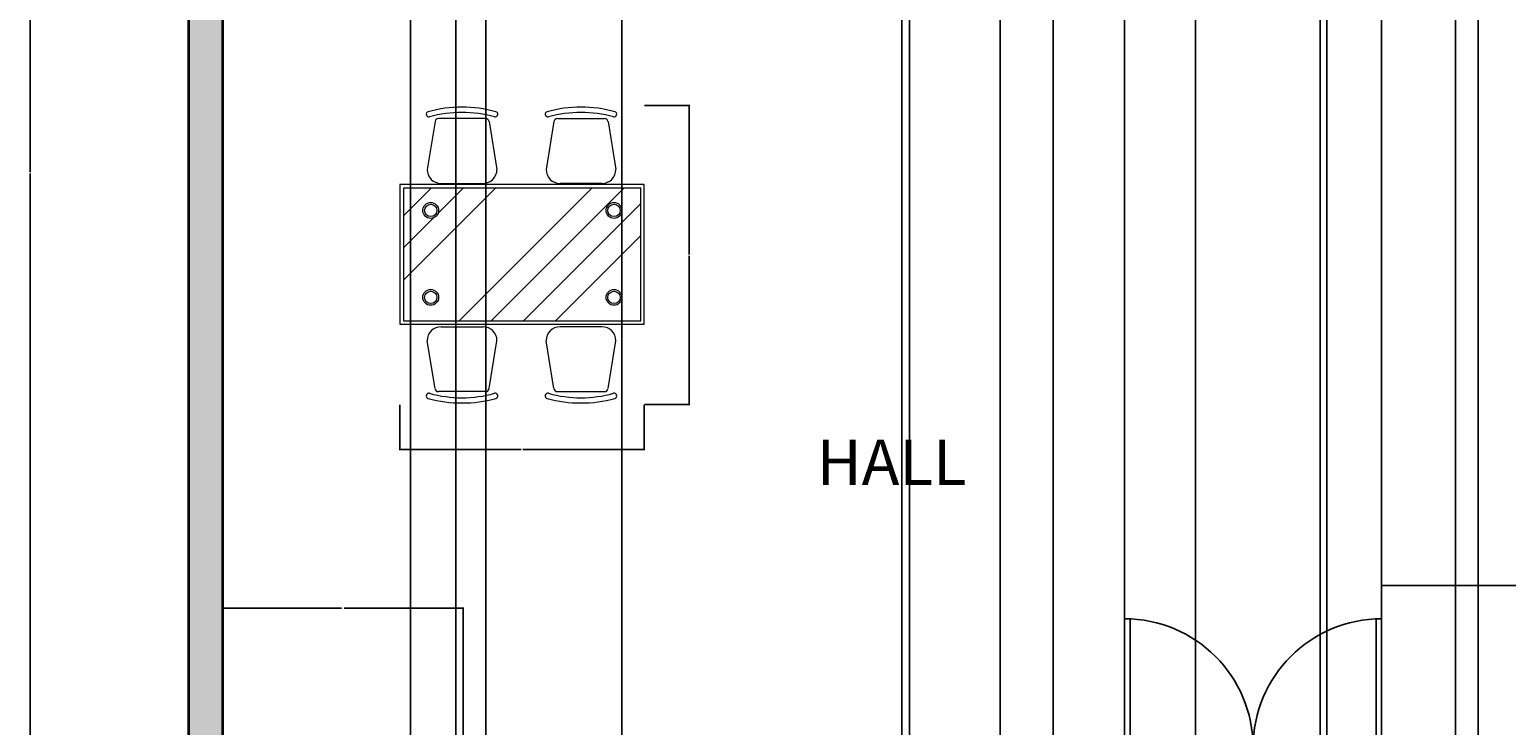
# Model space of a CAD drawing. Units: inches. Extents: x -89 to 661, y -827 to 77.
# Tile 2 of 5: x -44 to 347, y -523 to -339. Entities that reach past the tile are written whole.
import ezdxf

# ---------------------------------------------------------------- set-up
doc = ezdxf.new("R2010")
doc.units = ezdxf.units.IN
doc.header["$MEASUREMENT"] = 0
for name, color, linetype, lineweight in [('A-ANNO-DIMS', 2, 'Continuous', 18), ('A-AREA-IDEN', 7, 'Continuous', 18), ('A-FURN', 34, 'Continuous', 18), ('A-WALL', 7, 'Continuous', 35), ('A-WALL-PATT', 30, 'Continuous', 13), ('DOOR', 5, 'Continuous', 25)]:
    doc.layers.add(name, color=color, linetype=linetype, lineweight=lineweight)
doc.styles.get("Standard").update_dxf_attribs({"font": 'arial.ttf'})
doc.dimstyles.get("Standard").update_dxf_attribs({"dimtxt": 0.18, "dimasz": 0.18, "dimexe": 0.18, "dimexo": 0.0625, "dimgap": 0.09, "dimtad": 0, "dimtih": 1, "dimtoh": 1, "dimdec": 4, "dimzin": 0, "dimdsep": 46, "dimtxsty": 'Standard', "dimcen": 0.09, "dimadec": 0, "dimazin": 0, "dimtfac": 1, "dimtdec": 4, "dimtofl": 0, "dimtmove": 0, "dimatfit": 3, "dimfxl": 1, "dimtolj": 1, "dimtzin": 0, "dimarcsym": 0})

# ---------------------------------------------------------------- blocks, each defined once
blk = doc.blocks.new('*U7')
for p, q in [((0, 0), (0, -6)), ((40, 0), (40, -6))]:
    blk.add_line(p, q)
blk.add_lwpolyline([(0, 0), (0, 40), (1.75, 40), (1.75, 0)], close=True)
blk.add_arc((0, 0), 40, 0, 90)
blk = doc.blocks.new('A$C0FD55737')
for p, q in [((0.2013, 1.6134), (0.1562, 1.3384)), ((0.4912, 1.6302), (0.2211, 1.6302)), ((0.511, 1.6134), (0.5562, 1.3384)), ((0.8828, 1.6134), (0.8376, 1.3384)), ((0.9026, 1.6302), (1.1727, 1.6302)), ((1.1925, 1.6134), (1.2376, 1.3384)), ((0, 1.2513), (0, 0.4513)), ((1.4, 1.2513), (0, 1.2513)), ((0.02, 1.0725), (0.1788, 1.2313)), ((0.02, 0.7043), (0.547, 1.2313)), ((1.38, 1.2313), (0.02, 1.2313)), ((0.02, 1.2313), (0.02, 0.4713)), ((0.2189, 1.0873), (0.3629, 1.2313)), ((0.2362, 1.2584), (0.4762, 1.2584)), ((0.3393, 0.4713), (1.0993, 1.2313)), ((0.5234, 0.4713), (1.2834, 1.2313)), ((1.1576, 1.2584), (0.9176, 1.2584)), ((1.38, 0.4713), (1.38, 1.2313)), ((1.4, 0.4513), (1.4, 1.2513)), ((0.7074, 0.4713), (1.38, 1.1438)), ((0.02, 0.8884), (0.1931, 1.0614)), ((0.8915, 0.4713), (1.38, 0.9597)), ((0, 0.4513), (1.4, 0.4513)), ((0.02, 0.4713), (1.38, 0.4713)), ((0.2362, 0.4371), (0.4762, 0.4371)), ((1.1576, 0.4371), (0.9176, 0.4371)), ((0.2013, 0.0821), (0.1562, 0.3571)), ((0.511, 0.0821), (0.5562, 0.3571)), ((0.8828, 0.0821), (0.8376, 0.3571)), ((1.1925, 0.0821), (1.2376, 0.3571)), ((0.4912, 0.0653), (0.2211, 0.0653)), ((0.9026, 0.0653), (1.1727, 0.0653))]:
    blk.add_line(p, q)
for centre, radius in [((0.1766, 1.1037), 0.0454), ((0.1766, 1.1037), 0.0354), ((1.227, 1.1037), 0.0454), ((1.227, 1.1037), 0.0354), ((0.1766, 0.6052), 0.0454), ((0.1766, 0.6052), 0.0354), ((1.227, 0.6052), 0.0454), ((1.227, 0.6052), 0.0354)]:
    blk.add_circle(centre, radius)
for centre, radius, start, end in [((0.3562, 0.9712), 0.7243, 74.47014, 105.57697), ((1.0376, 0.9712), 0.7243, 74.42303, 105.52986), ((0.1662, 1.6546), 0.015, 105.49005, 284.28424), ((0.3562, 0.9716), 0.6939, 74.43245, 105.56755), ((0.2211, 1.6102), 0.02, 90, 170.67171), ((0.4912, 1.6102), 0.02, 9.32829, 90), ((0.5461, 1.6546), 0.015, 255.71576, 74.50995), ((0.8477, 1.6546), 0.015, 105.49005, 284.28424), ((1.0376, 0.9716), 0.6939, 74.43245, 105.56755), ((0.9026, 1.6102), 0.02, 90, 170.67171), ((1.1727, 1.6102), 0.02, 9.32829, 90), ((1.2276, 1.6546), 0.015, 255.71576, 74.50995), ((0.2362, 1.3384), 0.08, 180, 270), ((0.4762, 1.3384), 0.08, 270, 0), ((0.9176, 1.3384), 0.08, 180, 270), ((1.1576, 1.3384), 0.08, 270, 0), ((0.2362, 0.3571), 0.08, 90, 180), ((0.4762, 0.3571), 0.08, 0, 90), ((0.9176, 0.3571), 0.08, 90, 180), ((1.1576, 0.3571), 0.08, 0, 90), ((0.1662, 0.0409), 0.015, 75.71576, 254.50995), ((0.3562, 0.7243), 0.7243, 254.42303, 285.52986), ((0.3562, 0.7239), 0.6939, 254.43245, 285.56755), ((0.2211, 0.0853), 0.02, 189.32829, 270), ((0.4912, 0.0853), 0.02, 270, 350.67171), ((0.5461, 0.0409), 0.015, 285.49005, 104.28424), ((0.8477, 0.0409), 0.015, 75.71576, 254.50995), ((1.0376, 0.7243), 0.7243, 254.47014, 285.57697), ((1.0376, 0.7239), 0.6939, 254.43245, 285.56755), ((0.9026, 0.0853), 0.02, 189.32829, 270), ((1.1727, 0.0853), 0.02, 270, 350.67171), ((1.2276, 0.0409), 0.015, 285.49005, 104.28424)]:
    blk.add_arc(centre, radius, start, end)
blk = doc.blocks.new('*D25')
at = {"layer": 'A-ANNO-DIMS', "color": 0, "lineweight": -2, "transparency": 16777216}
for p, q in [((118.73, -359.12), (130.71, -359.12)), ((130.53, -359.3), (130.53, -398.47)), ((130.53, -438), (130.53, -398.84)), ((118.73, -438.18), (130.71, -438.18))]:
    blk.add_line(p, q, dxfattribs=at)
at = {"layer": 'A-ANNO-DIMS', "color": 0, "transparency": 16777216}
for points in [[(130.5, -359.3), (130.56, -359.3), (130.53, -359.12)], [(130.5, -438), (130.56, -438), (130.53, -438.18)]]:
    blk.add_solid(points, dxfattribs=at)
at = {"layer": 'Defpoints', "color": 0, "transparency": 16777216}
for p in [(118.67, -359.12), (130.53, -359.12), (118.67, -438.18)]:
    blk.add_point(p, dxfattribs=at)
at = {"layer": 'A-ANNO-DIMS', "color": 0, "transparency": 16777216, "insert": (130.53, -398.65), "char_height": 0.18, "attachment_point": 5}
blk.add_mtext('\\A1;DINING SET 79', dxfattribs=at)
blk = doc.blocks.new('*D26')
at = {"layer": 'A-ANNO-DIMS', "color": 0, "lineweight": -2, "transparency": 16777216}
for p, q in [((54.06, -438.25), (54.06, -450.22)), ((118.67, -438.25), (118.67, -450.22)), ((54.24, -450.04), (86.15, -450.04)), ((118.49, -450.04), (86.59, -450.04))]:
    blk.add_line(p, q, dxfattribs=at)
at = {"layer": 'A-ANNO-DIMS', "color": 0, "transparency": 16777216}
for points in [[(54.24, -450.01), (54.24, -450.07), (54.06, -450.04)], [(118.49, -450.01), (118.49, -450.07), (118.67, -450.04)]]:
    blk.add_solid(points, dxfattribs=at)
at = {"layer": 'Defpoints', "color": 0, "transparency": 16777216}
for p in [(54.06, -438.18), (118.67, -438.18), (118.67, -450.04)]:
    blk.add_point(p, dxfattribs=at)
at = {"layer": 'A-ANNO-DIMS', "color": 0, "transparency": 16777216, "insert": (86.37, -450.04), "char_height": 0.18, "attachment_point": 5}
blk.add_mtext('\\A1;65', dxfattribs=at)
blk = doc.blocks.new('*D32')
at = {"layer": 'A-ANNO-DIMS', "color": 0, "lineweight": -2, "transparency": 16777216}
for p, q in [((-1.88, 29.06), (-43.85, 29.06)), ((-43.67, 28.88), (-43.67, -376.76)), ((-43.67, -782.76), (-43.67, -377.12)), ((-1.88, -782.94), (-43.85, -782.94))]:
    blk.add_line(p, q, dxfattribs=at)
at = {"layer": 'A-ANNO-DIMS', "color": 0, "transparency": 16777216}
for points in [[(-43.7, 28.88), (-43.64, 28.88), (-43.67, 29.06)], [(-43.7, -782.76), (-43.64, -782.76), (-43.67, -782.94)]]:
    blk.add_solid(points, dxfattribs=at)
at = {"layer": 'Defpoints', "color": 0, "transparency": 16777216}
for p in [(-43.67, 29.06), (-1.81, 29.06), (-1.81, -782.94)]:
    blk.add_point(p, dxfattribs=at)
at = {"layer": 'A-ANNO-DIMS', "color": 0, "transparency": 16777216, "insert": (-43.67, -376.94), "char_height": 0.18, "attachment_point": 5}
blk.add_mtext('\\A1;812', dxfattribs=at)
blk = doc.blocks.new('*D44')
at = {"layer": 'A-ANNO-DIMS', "color": 0, "lineweight": -2, "transparency": 16777216}
for p, q in [((299.19, -34), (299.19, -826.85)), ((333.19, -34), (333.19, -826.85)), ((299.37, -826.67), (315.97, -826.67)), ((333.01, -826.67), (316.4, -826.67))]:
    blk.add_line(p, q, dxfattribs=at)
at = {"layer": 'A-ANNO-DIMS', "color": 0, "transparency": 16777216}
for points in [[(299.37, -826.64), (299.37, -826.7), (299.19, -826.67)], [(333.01, -826.64), (333.01, -826.7), (333.19, -826.67)]]:
    blk.add_solid(points, dxfattribs=at)
at = {"layer": 'Defpoints', "color": 0, "transparency": 16777216}
for p in [(299.19, -33.94), (333.19, -33.94), (333.19, -826.67)]:
    blk.add_point(p, dxfattribs=at)
at = {"layer": 'A-ANNO-DIMS', "color": 0, "transparency": 16777216, "insert": (316.19, -826.67), "char_height": 0.18, "attachment_point": 5}
blk.add_mtext('\\A1;34', dxfattribs=at)
blk = doc.blocks.new('*D46')
at = {"layer": 'A-ANNO-DIMS', "color": 0, "lineweight": -2, "transparency": 16777216}
for p, q in [((333.19, -34), (333.19, -826.85)), ((339.19, -34), (339.19, -826.85)), ((333.37, -826.67), (336.04, -826.67)), ((339.01, -826.67), (336.34, -826.67))]:
    blk.add_line(p, q, dxfattribs=at)
at = {"layer": 'A-ANNO-DIMS', "color": 0, "transparency": 16777216}
for points in [[(333.37, -826.64), (333.37, -826.7), (333.19, -826.67)], [(339.01, -826.64), (339.01, -826.7), (339.19, -826.67)]]:
    blk.add_solid(points, dxfattribs=at)
at = {"layer": 'Defpoints', "color": 0, "transparency": 16777216}
for p in [(333.19, -33.94), (339.19, -33.94), (339.19, -826.67)]:
    blk.add_point(p, dxfattribs=at)
at = {"layer": 'A-ANNO-DIMS', "color": 0, "transparency": 16777216, "insert": (336.19, -826.67), "char_height": 0.18, "attachment_point": 5}
blk.add_mtext('\\A1;6', dxfattribs=at)
blk = doc.blocks.new('*D48')
at = {"layer": 'A-ANNO-DIMS', "color": 0, "lineweight": -2, "transparency": 16777216}
for p, q in [((297.44, 2.03), (297.44, -826.85)), ((264.44, -8.47), (264.44, -826.85)), ((264.62, -826.67), (280.72, -826.67)), ((297.26, -826.67), (281.15, -826.67))]:
    blk.add_line(p, q, dxfattribs=at)
at = {"layer": 'A-ANNO-DIMS', "color": 0, "transparency": 16777216}
for points in [[(264.62, -826.64), (264.62, -826.7), (264.44, -826.67)], [(297.26, -826.64), (297.26, -826.7), (297.44, -826.67)]]:
    blk.add_solid(points, dxfattribs=at)
at = {"layer": 'Defpoints', "color": 0, "transparency": 16777216}
for p in [(297.44, 2.09), (264.44, -8.41), (297.44, -826.67)]:
    blk.add_point(p, dxfattribs=at)
at = {"layer": 'A-ANNO-DIMS', "color": 0, "transparency": 16777216, "insert": (280.94, -826.67), "char_height": 0.18, "attachment_point": 5}
blk.add_mtext('\\A1;33', dxfattribs=at)
blk = doc.blocks.new('*D55')
at = {"layer": 'A-ANNO-DIMS', "color": 0, "lineweight": -2, "transparency": 16777216}
for p, q in [((56.84, -267), (56.84, -826.85)), ((68.84, -267), (68.84, -826.85)), ((57.02, -826.67), (62.63, -826.67)), ((68.66, -826.67), (63.05, -826.67))]:
    blk.add_line(p, q, dxfattribs=at)
at = {"layer": 'A-ANNO-DIMS', "color": 0, "transparency": 16777216}
for points in [[(57.02, -826.64), (57.02, -826.7), (56.84, -826.67)], [(68.66, -826.64), (68.66, -826.7), (68.84, -826.67)]]:
    blk.add_solid(points, dxfattribs=at)
at = {"layer": 'Defpoints', "color": 0, "transparency": 16777216}
for p in [(56.84, -266.94), (68.84, -266.94), (68.84, -826.67)]:
    blk.add_point(p, dxfattribs=at)
at = {"layer": 'A-ANNO-DIMS', "color": 0, "transparency": 16777216, "insert": (62.84, -826.67), "char_height": 0.18, "attachment_point": 5}
blk.add_mtext('\\A1;12', dxfattribs=at)
blk = doc.blocks.new('*D56')
at = {"layer": 'A-ANNO-DIMS', "color": 0, "lineweight": -2, "transparency": 16777216}
for p, q in [((188.84, -312), (188.84, -826.85)), ((212.84, -318), (212.84, -826.85)), ((189.02, -826.67), (200.62, -826.67)), ((212.66, -826.67), (201.06, -826.67))]:
    blk.add_line(p, q, dxfattribs=at)
at = {"layer": 'A-ANNO-DIMS', "color": 0, "transparency": 16777216}
for points in [[(189.02, -826.64), (189.02, -826.7), (188.84, -826.67)], [(212.66, -826.64), (212.66, -826.7), (212.84, -826.67)]]:
    blk.add_solid(points, dxfattribs=at)
at = {"layer": 'Defpoints', "color": 0, "transparency": 16777216}
for p in [(188.84, -311.94), (212.84, -317.94), (212.84, -826.67)]:
    blk.add_point(p, dxfattribs=at)
at = {"layer": 'A-ANNO-DIMS', "color": 0, "transparency": 16777216, "insert": (200.84, -826.67), "char_height": 0.18, "attachment_point": 5}
blk.add_mtext('\\A1;24', dxfattribs=at)
blk = doc.blocks.new('*D61')
at = {"layer": 'A-ANNO-DIMS', "color": 0, "lineweight": -2, "transparency": 16777216}
for p, q in [((245.68, -494.78), (245.68, 77.13)), ((245.86, 76.95), (279.46, 76.95)), ((313.5, 76.95), (279.9, 76.95)), ((313.68, -494.78), (313.68, 77.13))]:
    blk.add_line(p, q, dxfattribs=at)
at = {"layer": 'A-ANNO-DIMS', "color": 0, "transparency": 16777216}
for points in [[(245.86, 76.98), (245.86, 76.92), (245.68, 76.95)], [(313.5, 76.98), (313.5, 76.92), (313.68, 76.95)]]:
    blk.add_solid(points, dxfattribs=at)
at = {"layer": 'Defpoints', "color": 0, "transparency": 16777216}
for p in [(313.68, 76.95), (245.68, -494.84), (313.68, -494.84)]:
    blk.add_point(p, dxfattribs=at)
at = {"layer": 'A-ANNO-DIMS', "color": 0, "transparency": 16777216, "insert": (279.68, 76.95), "char_height": 0.18, "attachment_point": 5}
blk.add_mtext('\\A1;68', dxfattribs=at)
blk = doc.blocks.new('*D62')
at = {"layer": 'A-ANNO-DIMS', "color": 0, "lineweight": -2, "transparency": 16777216}
for p, q in [((186.79, -527.88), (186.79, 77.13)), ((186.97, 76.95), (206.57, 76.95)), ((226.61, 76.95), (207.01, 76.95)), ((226.79, -527.88), (226.79, 77.13))]:
    blk.add_line(p, q, dxfattribs=at)
at = {"layer": 'A-ANNO-DIMS', "color": 0, "transparency": 16777216}
for points in [[(186.97, 76.98), (186.97, 76.92), (186.79, 76.95)], [(226.61, 76.98), (226.61, 76.92), (226.79, 76.95)]]:
    blk.add_solid(points, dxfattribs=at)
at = {"layer": 'Defpoints', "color": 0, "transparency": 16777216}
for p in [(226.79, 76.95), (186.79, -527.94), (226.79, -527.94)]:
    blk.add_point(p, dxfattribs=at)
at = {"layer": 'A-ANNO-DIMS', "color": 0, "transparency": 16777216, "insert": (206.79, 76.95), "char_height": 0.18, "attachment_point": 5}
blk.add_mtext('\\A1;40', dxfattribs=at)
blk = doc.blocks.new('*D63')
at = {"layer": 'A-ANNO-DIMS', "color": 0, "lineweight": -2, "transparency": 16777216}
for p, q in [((7.19, -533.88), (7.19, -491.9)), ((7.37, -492.08), (38.66, -492.08)), ((70.61, -492.08), (39.31, -492.08)), ((70.79, -533.88), (70.79, -491.9))]:
    blk.add_line(p, q, dxfattribs=at)
at = {"layer": 'A-ANNO-DIMS', "color": 0, "transparency": 16777216}
for points in [[(7.37, -492.05), (7.37, -492.11), (7.19, -492.08)], [(70.61, -492.05), (70.61, -492.11), (70.79, -492.08)]]:
    blk.add_solid(points, dxfattribs=at)
at = {"layer": 'Defpoints', "color": 0, "transparency": 16777216}
for p in [(70.79, -492.08), (7.19, -533.94), (70.79, -533.94)]:
    blk.add_point(p, dxfattribs=at)
at = {"layer": 'A-ANNO-DIMS', "color": 0, "transparency": 16777216, "insert": (38.99, -492.08), "char_height": 0.18, "attachment_point": 5}
blk.add_mtext('\\A1;63.6', dxfattribs=at)
blk = doc.blocks.new('*D69')
at = {"layer": 'A-ANNO-DIMS', "color": 0, "lineweight": -2, "transparency": 16777216}
for p, q in [((76.79, -629.88), (76.79, 77.13)), ((76.97, 76.95), (94.39, 76.95)), ((112.59, 76.95), (95.17, 76.95)), ((112.77, -629.88), (112.77, 77.13))]:
    blk.add_line(p, q, dxfattribs=at)
at = {"layer": 'A-ANNO-DIMS', "color": 0, "transparency": 16777216}
for points in [[(76.97, 76.98), (76.97, 76.92), (76.79, 76.95)], [(112.59, 76.98), (112.59, 76.92), (112.77, 76.95)]]:
    blk.add_solid(points, dxfattribs=at)
at = {"layer": 'Defpoints', "color": 0, "transparency": 16777216}
for p in [(112.77, 76.95), (76.79, -629.94), (112.77, -629.94)]:
    blk.add_point(p, dxfattribs=at)
at = {"layer": 'A-ANNO-DIMS', "color": 0, "transparency": 16777216, "insert": (94.78, 76.95), "char_height": 0.18, "attachment_point": 5}
blk.add_mtext('\\A1;35.98', dxfattribs=at)
blk = doc.blocks.new('*D74')
at = {"layer": 'A-ANNO-DIMS', "color": 0, "lineweight": -2, "transparency": 16777216}
for p, q in [((313.68, -527.88), (313.68, -485.9)), ((313.86, -486.08), (351.48, -486.08)), ((389.89, -486.08), (352.27, -486.08)), ((390.07, -527.88), (390.07, -485.9))]:
    blk.add_line(p, q, dxfattribs=at)
at = {"layer": 'A-ANNO-DIMS', "color": 0, "transparency": 16777216}
for points in [[(313.86, -486.05), (313.86, -486.11), (313.68, -486.08)], [(389.89, -486.05), (389.89, -486.11), (390.07, -486.08)]]:
    blk.add_solid(points, dxfattribs=at)
at = {"layer": 'Defpoints', "color": 0, "transparency": 16777216}
for p in [(390.07, -486.08), (313.68, -527.94), (390.07, -527.94)]:
    blk.add_point(p, dxfattribs=at)
at = {"layer": 'A-ANNO-DIMS', "color": 0, "transparency": 16777216, "insert": (351.88, -486.08), "char_height": 0.18, "attachment_point": 5}
blk.add_mtext('\\A1;76.39', dxfattribs=at)

msp = doc.modelspace()

# ---------------------------------------------------------------- hatches: boundary and pattern name
at = {"layer": 'A-WALL-PATT'}
h = msp.add_hatch(color=256, dxfattribs=at)
h.dxf.hatch_style = 1
h.paths.add_polyline_path([(255.186, 29.06), (-1.814, 29.06), (-1.814, -33.94), (7.186, -33.94), (7.186, -27.94), (7.186, 20.06), (255.186, 20.06)])
h.paths.add_polyline_path([(174.616, -27.94), (7.186, -27.94), (7.186, -33.94), (174.616, -33.94)], flags=17)
h.paths.add_polyline_path([(7.186, -33.94), (-1.814, -33.94), (-1.814, -527.94), (7.186, -527.94), (7.186, -425.94), (7.186, -311.94), (7.186, -207.94)])
h.paths.add_polyline_path([(7.186, -527.94), (-1.814, -527.94), (-1.814, -782.94), (430.186, -782.94), (430.186, -773.94), (7.186, -773.94)])

# ---------------------------------------------------------------- linework, layer by layer
at = {"layer": 'A-WALL'}
for p, q in [((-1.814, 29.06), (-1.814, -782.94)), ((7.186, -311.94), (7.186, -425.94)), ((7.186, -425.94), (7.186, -527.94))]:
    msp.add_line(p, q, dxfattribs=at)

# ---------------------------------------------------------------- block references
at = {"layer": 'A-FURN', "xscale": 46.14570200152887, "yscale": 46.14570200152887, "zscale": 46.14570200152887}
msp.add_blockref('A$C0FD55737', (54.064, -437.773), dxfattribs=at)
at = {"layer": 'DOOR', "yscale": 0.85, "zscale": 0.85}
for p, xscale in [((245.682, -528.84), 0.85), ((313.682, -528.84), -0.85)]:
    msp.add_blockref('*U7', p, dxfattribs=dict(at, xscale=xscale))

# ---------------------------------------------------------------- texts
at = {"layer": 'A-AREA-IDEN', "insert": (155.948, -447.43), "char_height": 12, "attachment_point": 1}
msp.add_mtext_dynamic_manual_height_columns('\\pxqc;{\\fArial|b1|i0|c0|p34;HALL}', width=56.29646, gutter_width=1, heights=[0], dxfattribs=at)

# ---------------------------------------------------------------- dimensions: what is measured, and where the dimension line sits
at = {"layer": 'A-ANNO-DIMS'}
for base, p1, p2, override, picture, middle in [((112.77, 76.952), (76.788, -629.94), (112.77, -629.94), {"dimdec": 2, "dimlfac": 1, "dimrnd": 0, "dimzin": 0, "dimdsep": 46, "dimlunit": 2}, '*D69', (94.779, 76.952)), ((226.788, 76.952), (186.788, -527.94), (226.788, -527.94), {"dimdec": 0, "dimlfac": 1, "dimrnd": 0, "dimzin": 0, "dimdsep": 46, "dimlunit": 2}, '*D62', (206.788, 76.952)), ((313.682, 76.952), (245.682, -494.84), (313.682, -494.84), {"dimdec": 0, "dimlfac": 1, "dimrnd": 0, "dimzin": 0, "dimdsep": 46, "dimlunit": 2}, '*D61', (279.682, 76.952)), ((297.436, -826.669), (264.436, -8.408), (297.436, 2.092), {"dimdec": 0, "dimlfac": 1, "dimrnd": 0, "dimzin": 0, "dimdsep": 46, "dimlunit": 2}, '*D48', (280.936, -826.669)), ((333.186, -826.669), (299.186, -33.94), (333.186, -33.94), {"dimdec": 0, "dimlfac": 1, "dimrnd": 0, "dimzin": 0, "dimdsep": 46, "dimlunit": 2}, '*D44', (316.186, -826.669)), ((339.186, -826.669), (333.186, -33.94), (339.186, -33.94), {"dimdec": 0, "dimlfac": 1, "dimrnd": 0, "dimzin": 0, "dimdsep": 46, "dimlunit": 2}, '*D46', (336.186, -826.669)), ((68.837, -826.669), (56.837, -266.94), (68.837, -266.94), {"dimdec": 0, "dimlfac": 1, "dimrnd": 0, "dimzin": 0, "dimdsep": 46, "dimlunit": 2}, '*D55', (62.837, -826.669)), ((212.837, -826.669), (188.837, -311.94), (212.837, -317.94), {"dimdec": 0, "dimlfac": 1, "dimrnd": 0, "dimzin": 0, "dimdsep": 46, "dimlunit": 2}, '*D56', (200.837, -826.669)), ((118.668, -450.042), (54.064, -438.183), (118.668, -438.183), {"dimdec": 0, "dimlfac": 1, "dimrnd": 0, "dimzin": 0, "dimdsep": 46, "dimlunit": 2}, '*D26', (86.366, -450.042)), ((390.071, -486.08), (313.682, -527.94), (390.071, -527.94), {"dimdec": 2, "dimlfac": 1, "dimrnd": 0, "dimzin": 0, "dimdsep": 46, "dimlunit": 2}, '*D74', (351.876, -486.08)), ((70.788, -492.08), (7.186, -533.94), (70.788, -533.94), {"dimdec": 1, "dimlfac": 1, "dimrnd": 0, "dimzin": 0, "dimdsep": 46, "dimlunit": 2}, '*D63', (38.987, -492.08))]:
    dim = msp.add_linear_dim(base=base, p1=p1, p2=p2, dimstyle='Standard', override=override, dxfattribs=at)
    dim.commit()
    dim.dimension.update_dxf_attribs({"geometry": picture, "text_midpoint": middle})
dim = msp.add_linear_dim(base=(-43.674, 29.06), p1=(-1.814, -782.94), p2=(-1.814, 29.06), angle=90, dimstyle='Standard', override={"dimdec": 0, "dimlfac": 1, "dimrnd": 0, "dimzin": 0, "dimdsep": 46, "dimlunit": 2}, dxfattribs=at)
dim.commit()
dim.dimension.update_dxf_attribs({"geometry": '*D32', "text_midpoint": (-43.674, -376.94)})
dim = msp.add_linear_dim(base=(130.526, -359.124), p1=(118.668, -438.183), p2=(118.668, -359.124), angle=90, text='DINING SET <>', dimstyle='Standard', override={"dimdec": 0, "dimlfac": 1, "dimrnd": 0, "dimzin": 0, "dimdsep": 46, "dimlunit": 2}, dxfattribs=at)
dim.commit()
dim.dimension.update_dxf_attribs({"geometry": '*D25', "text_midpoint": (130.526, -398.653)})

doc.saveas('drawing.dxf')
